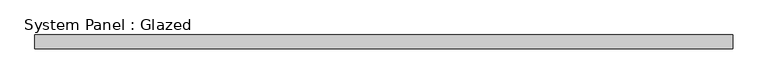
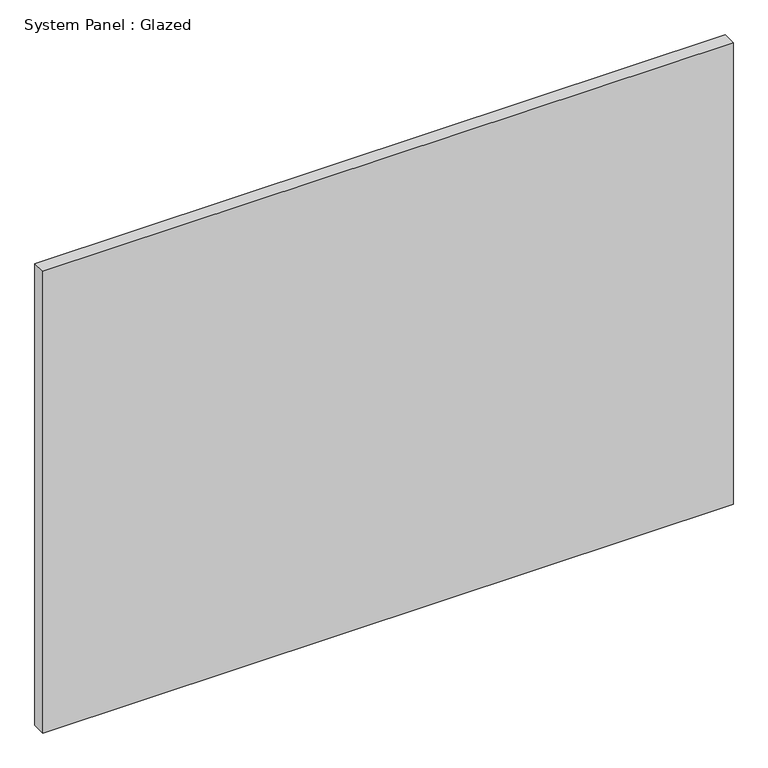
"""IFC4 building model written with IfcOpenShell, lengths in millimetres: plate geometry, System Panel : Glazed."""

from ifc_helpers import new_model, si_unit, origin, origin_with_axes, place, context, project, spatial, polyline, outline, extrude, source, transform, mapped, element, save


def system_panel_glazed_b72ced83(model_context):
    return source(origin(), model_context, "Body", "SweptSolid", [
        extrude(outline(polyline([(650.8750001, -44.45), (-650.8750001, -44.45), (-650.8750001, -19.05), (650.8750001, -19.05), (650.8750001, -44.45)])), origin_with_axes(), (0.0, 0.0, 1.0), 920.75),
    ])


if __name__ == "__main__":
    model = new_model("IFC4")
    model_context = context("Model", 3, world=origin())
    ifc_project = project(units=[si_unit("LENGTHUNIT", "METRE", prefix="MILLI")], contexts=[model_context])
    site = spatial("IfcSite", under=ifc_project)
    building = spatial("IfcBuilding", under=site)
    placement = place(None, origin())
    system_panel_glazed_shape = system_panel_glazed_b72ced83(model_context)
    element("IfcPlate", 1, ObjectType="System Panel : Glazed", at=placement, inside=building, context=model_context, shape_type="MappedRepresentation", body=[
        mapped(system_panel_glazed_shape, transform((0.0, 0.0, 0.0), x_axis=(1.0, 0.0, 0.0), y_axis=(0.0, 1.0, 0.0), z_axis=(0.0, 0.0, 1.0))),
    ])
    save(model, "model.ifc")

# Revit data of these elements
# Type "System Panel : Glazed"
#   Construction Type Id = "GSP4R"
#   Analytic Construction = "1/8 in Pilkington single glazing"
#   Visual Light Transmittance = 0.9
#   Solar Heat Gain Coefficient = 0.86
#   Heat Transfer Coefficient (U) = 1.18115 BTU/(h·ft²·°F)
#   Define Thermal Properties by = 1
# Element 1 (IfcPlate, "System Panel : Glazed")
#   Materials on its faces: "glass panel 223"
# Materials
#   "glass panel 223": class "Generic", colour RGB 120 120 120, transparency 0, Cost = 0
